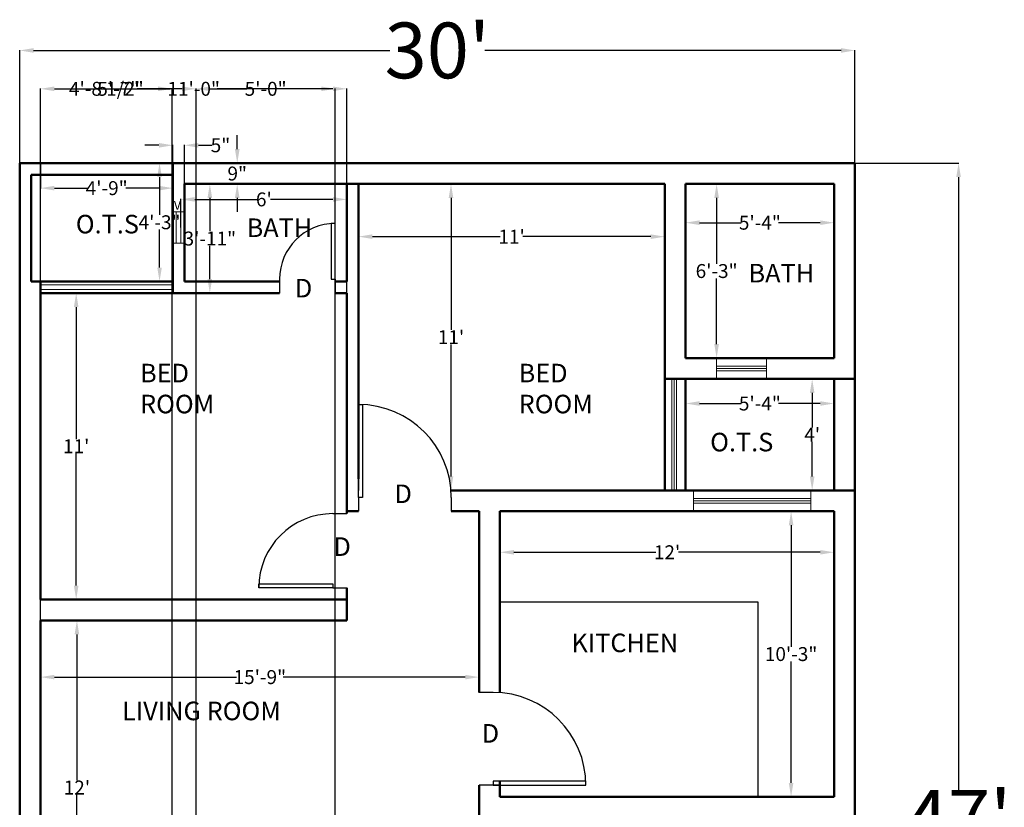
# Model space of a CAD drawing. Units: inches. Extents: x -251 to 272, y 511 to 1173.
# Tile 2 of 2: x -210 to 215, y 834 to 1173. Entities that reach past the tile are written whole.
import ezdxf

# ---------------------------------------------------------------- set-up
doc = ezdxf.new("R2010")
doc.units = ezdxf.units.IN
doc.header["$MEASUREMENT"] = 0
doc.layers.get('0').update_dxf_attribs({"color": 3})
for name, color, linetype, lineweight in [('A-AREA-IDEN', 20, 'Continuous', 25), ('A-FLOR-FIXT', 8, 'Continuous', 25), ('A-WALL', 7, 'Continuous', 50), ('dim', 2, 'Continuous', 18), ('door', 1, 'Continuous', 25), ('text', 20, 'Continuous', 18), ('window', 6, 'Continuous', 18)]:
    doc.layers.add(name, color=color, linetype=linetype, lineweight=lineweight)
doc.styles.get("Standard").update_dxf_attribs({"font": 'arial.ttf'})
doc.dimstyles.get("Standard").update_dxf_attribs({"dimtxt": 6, "dimasz": 6, "dimexe": 0.18, "dimexo": 0.0625, "dimgap": 0.09, "dimtad": 0, "dimtih": 1, "dimtoh": 1, "dimdec": 0, "dimzin": 0, "dimdsep": 46, "dimlunit": 3, "dimtxsty": 'Standard', "dimcen": 0.09, "dimadec": 0, "dimazin": 0, "dimtfac": 1, "dimtdec": 0, "dimtofl": 0, "dimtmove": 0, "dimatfit": 3, "dimfxl": 1, "dimtolj": 1, "dimtzin": 0, "dimarcsym": 0})

# ---------------------------------------------------------------- blocks, each defined once
blk = doc.blocks.new('*U2')
for p, q in [((-24, 0), (-24, -6)), ((0, 0), (0, -6))]:
    blk.add_line(p, q)
blk.add_lwpolyline([(0, 0), (0, 24), (-1.75, 24), (-1.75, 0)], close=True)
blk.add_arc((0, 0), 24, 90, 180)
blk = doc.blocks.new('*D3')
at = {"layer": 'Defpoints', "color": 0, "transparency": 16777216}
for p in [(-143.69, 1111.09), (-149.41, 1060.09), (-143.69, 1060.09)]:
    blk.add_point(p, dxfattribs=at)
at = {"layer": 'dim', "color": 0, "lineweight": -2, "transparency": 16777216}
for p, q in [((-143.75, 1111.09), (-149.59, 1111.09)), ((-149.41, 1105.09), (-149.41, 1088.74)), ((-149.41, 1066.09), (-149.41, 1082.43)), ((-143.75, 1060.09), (-149.59, 1060.09))]:
    blk.add_line(p, q, dxfattribs=at)
at = {"layer": 'dim', "color": 0, "transparency": 16777216}
for points in [[(-150.41, 1105.09), (-148.41, 1105.09), (-149.41, 1111.09)], [(-150.41, 1066.09), (-148.41, 1066.09), (-149.41, 1060.09)]]:
    blk.add_solid(points, dxfattribs=at)
at = {"layer": 'dim', "color": 0, "transparency": 16777216, "insert": (-149.41, 1085.59), "char_height": 6, "attachment_point": 5}
blk.add_mtext('\\A1;4\'-3"', dxfattribs=at)
blk = doc.blocks.new('*D4')
at = {"layer": 'Defpoints', "color": 0, "transparency": 16777216}
for p in [(-200.69, 1111.09), (-143.69, 1111.09), (-143.69, 1100.3)]:
    blk.add_point(p, dxfattribs=at)
at = {"layer": 'dim', "color": 0, "lineweight": -2, "transparency": 16777216}
for p, q in [((-200.69, 1111.02), (-200.69, 1100.12)), ((-143.69, 1111.02), (-143.69, 1100.12)), ((-194.69, 1100.3), (-180.37, 1100.3)), ((-149.69, 1100.3), (-164, 1100.3))]:
    blk.add_line(p, q, dxfattribs=at)
at = {"layer": 'dim', "color": 0, "transparency": 16777216}
for points in [[(-194.69, 1101.3), (-194.69, 1099.3), (-200.69, 1100.3)], [(-149.69, 1101.3), (-149.69, 1099.3), (-143.69, 1100.3)]]:
    blk.add_solid(points, dxfattribs=at)
at = {"layer": 'dim', "color": 0, "transparency": 16777216, "insert": (-172.19, 1100.3), "char_height": 6, "attachment_point": 5}
blk.add_mtext('\\A1;4\'-9"', dxfattribs=at)
blk = doc.blocks.new('*D5')
at = {"layer": 'Defpoints', "color": 0, "transparency": 16777216}
for p in [(-138.69, 1118.76), (-143.69, 1100.12), (-138.69, 1100.12)]:
    blk.add_point(p, dxfattribs=at)
at = {"layer": 'dim', "color": 0, "lineweight": -2, "transparency": 16777216}
for p, q in [((-149.69, 1118.76), (-155.69, 1118.76)), ((-143.69, 1100.19), (-143.69, 1118.94)), ((-138.69, 1100.19), (-138.69, 1118.94)), ((-132.69, 1118.76), (-126.69, 1118.76))]:
    blk.add_line(p, q, dxfattribs=at)
at = {"layer": 'dim', "color": 0, "transparency": 16777216}
for points in [[(-149.69, 1119.76), (-149.69, 1117.76), (-143.69, 1118.76)], [(-132.69, 1119.76), (-132.69, 1117.76), (-138.69, 1118.76)]]:
    blk.add_solid(points, dxfattribs=at)
at = {"layer": 'dim', "color": 0, "transparency": 16777216, "insert": (-123.15, 1118.76), "char_height": 6, "attachment_point": 5}
blk.add_mtext('\\A1;5"', dxfattribs=at)
blk = doc.blocks.new('*D6')
at = {"layer": 'Defpoints', "color": 0, "transparency": 16777216}
for p in [(-125.07, 1111.09), (-124.46, 1102.09), (-115.93, 1102.09)]:
    blk.add_point(p, dxfattribs=at)
at = {"layer": 'dim', "color": 0, "lineweight": -2, "transparency": 16777216}
for p, q in [((-115.93, 1117.09), (-115.93, 1123.09)), ((-125, 1111.09), (-115.75, 1111.09)), ((-124.39, 1102.09), (-115.75, 1102.09)), ((-115.93, 1096.09), (-115.93, 1090.09))]:
    blk.add_line(p, q, dxfattribs=at)
at = {"layer": 'dim', "color": 0, "transparency": 16777216}
for points in [[(-116.93, 1117.09), (-114.93, 1117.09), (-115.93, 1111.09)], [(-116.93, 1096.09), (-114.93, 1096.09), (-115.93, 1102.09)]]:
    blk.add_solid(points, dxfattribs=at)
at = {"layer": 'dim', "color": 0, "transparency": 16777216, "insert": (-115.93, 1106.59), "char_height": 6, "attachment_point": 5}
blk.add_mtext('\\A1;9"', dxfattribs=at)
blk = doc.blocks.new('*D7')
at = {"layer": 'Defpoints', "color": 0, "transparency": 16777216}
for p in [(-200.69, 1055.09), (-200.69, 923.09), (-185.34, 923.09)]:
    blk.add_point(p, dxfattribs=at)
at = {"layer": 'dim', "color": 0, "lineweight": -2, "transparency": 16777216}
for p, q in [((-200.63, 1055.09), (-185.16, 1055.09)), ((-185.34, 1049.09), (-185.34, 992.19)), ((-185.34, 929.09), (-185.34, 985.99)), ((-200.63, 923.09), (-185.16, 923.09))]:
    blk.add_line(p, q, dxfattribs=at)
at = {"layer": 'dim', "color": 0, "transparency": 16777216}
for points in [[(-186.34, 1049.09), (-184.34, 1049.09), (-185.34, 1055.09)], [(-186.34, 929.09), (-184.34, 929.09), (-185.34, 923.09)]]:
    blk.add_solid(points, dxfattribs=at)
at = {"layer": 'dim', "color": 0, "transparency": 16777216, "insert": (-185.34, 989.09), "char_height": 6, "attachment_point": 5}
blk.add_mtext("\\A1;11'", dxfattribs=at)
blk = doc.blocks.new('*U12')
for p, q in [((0, 0), (0, -6)), ((32, 0), (32, -6))]:
    blk.add_line(p, q)
blk.add_lwpolyline([(0, 0), (0, 32), (1.75, 32), (1.75, 0)], close=True)
blk.add_arc((0, 0), 32, 0, 90)
blk = doc.blocks.new('*U8')
for p, q in [((0, 0), (0, -6)), ((40, 0), (40, -6))]:
    blk.add_line(p, q)
blk.add_lwpolyline([(0, 0), (0, 40), (1.75, 40), (1.75, 0)], close=True)
blk.add_arc((0, 0), 40, 0, 90)
blk = doc.blocks.new('*D9')
at = {"layer": 'Defpoints', "color": 0, "transparency": 16777216}
for p in [(-68.69, 1095.45), (-140.22, 1083.32), (-68.69, 1083.32)]:
    blk.add_point(p, dxfattribs=at)
at = {"layer": 'dim', "color": 0, "lineweight": -2, "transparency": 16777216}
for p, q in [((-140.22, 1083.38), (-140.22, 1095.63)), ((-134.22, 1095.45), (-107.32, 1095.45)), ((-74.69, 1095.45), (-101.59, 1095.45)), ((-68.69, 1083.38), (-68.69, 1095.63))]:
    blk.add_line(p, q, dxfattribs=at)
at = {"layer": 'dim', "color": 0, "transparency": 16777216}
for points in [[(-134.22, 1096.45), (-134.22, 1094.45), (-140.22, 1095.45)], [(-74.69, 1096.45), (-74.69, 1094.45), (-68.69, 1095.45)]]:
    blk.add_solid(points, dxfattribs=at)
at = {"layer": 'dim', "color": 0, "transparency": 16777216, "insert": (-104.46, 1095.45), "char_height": 6, "attachment_point": 5}
blk.add_mtext("\\A1;6'", dxfattribs=at)
blk = doc.blocks.new('*D10')
at = {"layer": 'Defpoints', "color": 0, "transparency": 16777216}
for p in [(-127.74, 1102.09), (-127.74, 1102.09), (-127.74, 1055.09)]:
    blk.add_point(p, dxfattribs=at)
at = {"layer": 'dim', "color": 0, "lineweight": -2, "transparency": 16777216}
for p, q in [((-127.8, 1102.09), (-127.92, 1102.09)), ((-127.74, 1096.09), (-127.74, 1081.74)), ((-127.74, 1061.09), (-127.74, 1075.43)), ((-127.8, 1055.09), (-127.92, 1055.09))]:
    blk.add_line(p, q, dxfattribs=at)
at = {"layer": 'dim', "color": 0, "transparency": 16777216}
for points in [[(-128.74, 1096.09), (-126.74, 1096.09), (-127.74, 1102.09)], [(-128.74, 1061.09), (-126.74, 1061.09), (-127.74, 1055.09)]]:
    blk.add_solid(points, dxfattribs=at)
at = {"layer": 'dim', "color": 0, "transparency": 16777216, "insert": (-127.74, 1078.59), "char_height": 6, "attachment_point": 5}
blk.add_mtext('\\A1;3\'-11"', dxfattribs=at)
blk = doc.blocks.new('*D11')
at = {"layer": 'Defpoints', "color": 0, "transparency": 16777216}
for p in [(-63.69, 1102.09), (68.31, 1102.09), (68.31, 1079.4)]:
    blk.add_point(p, dxfattribs=at)
at = {"layer": 'dim', "color": 0, "lineweight": -2, "transparency": 16777216}
for p, q in [((-63.69, 1102.02), (-63.69, 1079.22)), ((68.31, 1102.02), (68.31, 1079.22)), ((-57.69, 1079.4), (-2.59, 1079.4)), ((62.31, 1079.4), (7.21, 1079.4))]:
    blk.add_line(p, q, dxfattribs=at)
at = {"layer": 'dim', "color": 0, "transparency": 16777216}
for points in [[(-57.69, 1080.4), (-57.69, 1078.4), (-63.69, 1079.4)], [(62.31, 1080.4), (62.31, 1078.4), (68.31, 1079.4)]]:
    blk.add_solid(points, dxfattribs=at)
at = {"layer": 'dim', "color": 0, "transparency": 16777216, "insert": (2.31, 1079.4), "char_height": 6, "attachment_point": 5}
blk.add_mtext("\\A1;11'", dxfattribs=at)
blk = doc.blocks.new('*D13')
at = {"layer": 'Defpoints', "color": 0, "transparency": 16777216}
for p in [(-0.19, 1102.09), (-23.8, 970.09), (-0.19, 970.09)]:
    blk.add_point(p, dxfattribs=at)
at = {"layer": 'dim', "color": 0, "lineweight": -2, "transparency": 16777216}
for p, q in [((-0.25, 1102.09), (-23.98, 1102.09)), ((-23.8, 1096.09), (-23.8, 1039.19)), ((-23.8, 976.09), (-23.8, 1032.99)), ((-0.25, 970.09), (-23.98, 970.09))]:
    blk.add_line(p, q, dxfattribs=at)
at = {"layer": 'dim', "color": 0, "transparency": 16777216}
for points in [[(-24.8, 1096.09), (-22.8, 1096.09), (-23.8, 1102.09)], [(-24.8, 976.09), (-22.8, 976.09), (-23.8, 970.09)]]:
    blk.add_solid(points, dxfattribs=at)
at = {"layer": 'dim', "color": 0, "transparency": 16777216, "insert": (-23.8, 1036.09), "char_height": 6, "attachment_point": 5}
blk.add_mtext("\\A1;11'", dxfattribs=at)
blk = doc.blocks.new('*D14')
at = {"layer": 'Defpoints', "color": 0, "transparency": 16777216}
for p in [(77.31, 1102.09), (77.31, 1027.09), (90.67, 1027.09)]:
    blk.add_point(p, dxfattribs=at)
at = {"layer": 'dim', "color": 0, "lineweight": -2, "transparency": 16777216}
for p, q in [((77.37, 1102.09), (90.85, 1102.09)), ((90.67, 1096.09), (90.67, 1067.74)), ((90.67, 1033.09), (90.67, 1061.43)), ((77.37, 1027.09), (90.85, 1027.09))]:
    blk.add_line(p, q, dxfattribs=at)
at = {"layer": 'dim', "color": 0, "transparency": 16777216}
for points in [[(89.67, 1096.09), (91.67, 1096.09), (90.67, 1102.09)], [(89.67, 1033.09), (91.67, 1033.09), (90.67, 1027.09)]]:
    blk.add_solid(points, dxfattribs=at)
at = {"layer": 'dim', "color": 0, "transparency": 16777216, "insert": (90.67, 1064.59), "char_height": 6, "attachment_point": 5}
blk.add_mtext('\\A1;6\'-3"', dxfattribs=at)
blk = doc.blocks.new('*D15')
at = {"layer": 'Defpoints', "color": 0, "transparency": 16777216}
for p in [(77.31, 1102.09), (141.31, 1102.09), (77.31, 1085.41)]:
    blk.add_point(p, dxfattribs=at)
at = {"layer": 'dim', "color": 0, "lineweight": -2, "transparency": 16777216}
for p, q in [((77.31, 1102.02), (77.31, 1085.23)), ((141.31, 1102.02), (141.31, 1085.23)), ((83.31, 1085.41), (101.25, 1085.41)), ((135.31, 1085.41), (117.38, 1085.41))]:
    blk.add_line(p, q, dxfattribs=at)
at = {"layer": 'dim', "color": 0, "transparency": 16777216}
for points in [[(83.31, 1086.41), (83.31, 1084.41), (77.31, 1085.41)], [(135.31, 1086.41), (135.31, 1084.41), (141.31, 1085.41)]]:
    blk.add_solid(points, dxfattribs=at)
at = {"layer": 'dim', "color": 0, "transparency": 16777216, "insert": (109.31, 1085.41), "char_height": 6, "attachment_point": 5}
blk.add_mtext('\\A1;5\'-4"', dxfattribs=at)
blk = doc.blocks.new('*D16')
at = {"layer": 'Defpoints', "color": 0, "transparency": 16777216}
for p in [(77.31, 1018.09), (141.31, 1018.09), (77.31, 1007.53)]:
    blk.add_point(p, dxfattribs=at)
at = {"layer": 'dim', "color": 0, "lineweight": -2, "transparency": 16777216}
for p, q in [((77.31, 1018.02), (77.31, 1007.35)), ((141.31, 1018.02), (141.31, 1007.35)), ((83.31, 1007.53), (101.25, 1007.53)), ((135.31, 1007.53), (117.38, 1007.53))]:
    blk.add_line(p, q, dxfattribs=at)
at = {"layer": 'dim', "color": 0, "transparency": 16777216}
for points in [[(83.31, 1008.53), (83.31, 1006.53), (77.31, 1007.53)], [(135.31, 1008.53), (135.31, 1006.53), (141.31, 1007.53)]]:
    blk.add_solid(points, dxfattribs=at)
at = {"layer": 'dim', "color": 0, "transparency": 16777216, "insert": (109.31, 1007.53), "char_height": 6, "attachment_point": 5}
blk.add_mtext('\\A1;5\'-4"', dxfattribs=at)
blk = doc.blocks.new('*D17')
at = {"layer": 'Defpoints', "color": 0, "transparency": 16777216}
for p in [(131.85, 1018.09), (141.31, 1018.09), (141.31, 970.09)]:
    blk.add_point(p, dxfattribs=at)
at = {"layer": 'dim', "color": 0, "lineweight": -2, "transparency": 16777216}
for p, q in [((141.25, 1018.09), (131.67, 1018.09)), ((131.85, 1012.09), (131.85, 997.18)), ((131.85, 976.09), (131.85, 991)), ((141.25, 970.09), (131.67, 970.09))]:
    blk.add_line(p, q, dxfattribs=at)
at = {"layer": 'dim', "color": 0, "transparency": 16777216}
for points in [[(130.85, 1012.09), (132.85, 1012.09), (131.85, 1018.09)], [(130.85, 976.09), (132.85, 976.09), (131.85, 970.09)]]:
    blk.add_solid(points, dxfattribs=at)
at = {"layer": 'dim', "color": 0, "transparency": 16777216, "insert": (131.85, 994.09), "char_height": 6, "attachment_point": 5}
blk.add_mtext("\\A1;4'", dxfattribs=at)
blk = doc.blocks.new('*U18')
for p, q in [((0, 0), (0, 6)), ((40, 0), (40, 6))]:
    blk.add_line(p, q)
blk.add_lwpolyline([(0, 0), (0, -40), (1.75, -40), (1.75, 0)], close=True)
blk.add_arc((0, 0), 40, 270, 0)
blk = doc.blocks.new('*D19')
at = {"layer": 'Defpoints', "color": 0, "transparency": 16777216}
for p in [(141.31, 961.09), (122.77, 838.09), (141.31, 838.09)]:
    blk.add_point(p, dxfattribs=at)
at = {"layer": 'dim', "color": 0, "lineweight": -2, "transparency": 16777216}
for p, q in [((141.25, 961.09), (122.59, 961.09)), ((122.77, 955.09), (122.77, 902.74)), ((122.77, 844.09), (122.77, 896.43)), ((141.25, 838.09), (122.59, 838.09))]:
    blk.add_line(p, q, dxfattribs=at)
at = {"layer": 'dim', "color": 0, "transparency": 16777216}
for points in [[(121.77, 955.09), (123.77, 955.09), (122.77, 961.09)], [(121.77, 844.09), (123.77, 844.09), (122.77, 838.09)]]:
    blk.add_solid(points, dxfattribs=at)
at = {"layer": 'dim', "color": 0, "transparency": 16777216, "insert": (122.77, 899.59), "char_height": 6, "attachment_point": 5}
blk.add_mtext('\\A1;10\'-3"', dxfattribs=at)
blk = doc.blocks.new('*D20')
at = {"layer": 'Defpoints', "color": 0, "transparency": 16777216}
for p in [(-2.69, 961.09), (141.31, 961.09), (141.31, 943.44)]:
    blk.add_point(p, dxfattribs=at)
at = {"layer": 'dim', "color": 0, "lineweight": -2, "transparency": 16777216}
for p, q in [((-2.69, 961.02), (-2.69, 943.26)), ((141.31, 961.02), (141.31, 943.26)), ((3.31, 943.44), (64.41, 943.44)), ((135.31, 943.44), (74.21, 943.44))]:
    blk.add_line(p, q, dxfattribs=at)
at = {"layer": 'dim', "color": 0, "transparency": 16777216}
for points in [[(3.31, 944.44), (3.31, 942.44), (-2.69, 943.44)], [(135.31, 944.44), (135.31, 942.44), (141.31, 943.44)]]:
    blk.add_solid(points, dxfattribs=at)
at = {"layer": 'dim', "color": 0, "transparency": 16777216, "insert": (69.31, 943.44), "char_height": 6, "attachment_point": 5}
blk.add_mtext("\\A1;12'", dxfattribs=at)
blk = doc.blocks.new('*D36')
at = {"layer": 'Defpoints', "color": 0, "transparency": 16777216}
for p in [(-200.69, 914.09), (-200.69, 770.09), (-185.02, 770.09)]:
    blk.add_point(p, dxfattribs=at)
at = {"layer": 'dim', "color": 0, "lineweight": -2, "transparency": 16777216}
for p, q in [((-200.63, 914.09), (-184.84, 914.09)), ((-185.02, 908.09), (-185.02, 845.19)), ((-185.02, 776.09), (-185.02, 838.99)), ((-200.63, 770.09), (-184.84, 770.09))]:
    blk.add_line(p, q, dxfattribs=at)
at = {"layer": 'dim', "color": 0, "transparency": 16777216}
for points in [[(-186.02, 908.09), (-184.02, 908.09), (-185.02, 914.09)], [(-186.02, 776.09), (-184.02, 776.09), (-185.02, 770.09)]]:
    blk.add_solid(points, dxfattribs=at)
at = {"layer": 'dim', "color": 0, "transparency": 16777216, "insert": (-185.02, 842.09), "char_height": 6, "attachment_point": 5}
blk.add_mtext("\\A1;12'", dxfattribs=at)
blk = doc.blocks.new('*D37')
at = {"layer": 'Defpoints', "color": 0, "transparency": 16777216}
for p in [(-200.69, 914.09), (-11.69, 914.09), (-11.69, 889.67)]:
    blk.add_point(p, dxfattribs=at)
at = {"layer": 'dim', "color": 0, "lineweight": -2, "transparency": 16777216}
for p, q in [((-200.69, 914.02), (-200.69, 889.49)), ((-11.69, 914.02), (-11.69, 889.49)), ((-194.69, 889.67), (-116.3, 889.67)), ((-17.69, 889.67), (-96.07, 889.67))]:
    blk.add_line(p, q, dxfattribs=at)
at = {"layer": 'dim', "color": 0, "transparency": 16777216}
for points in [[(-194.69, 890.67), (-194.69, 888.67), (-200.69, 889.67)], [(-17.69, 890.67), (-17.69, 888.67), (-11.69, 889.67)]]:
    blk.add_solid(points, dxfattribs=at)
at = {"layer": 'dim', "color": 0, "transparency": 16777216, "insert": (-106.19, 889.67), "char_height": 6, "attachment_point": 5}
blk.add_mtext('\\A1;15\'-9"', dxfattribs=at)
blk = doc.blocks.new('*D38')
at = {"layer": 'Defpoints', "color": 0, "transparency": 16777216}
for p in [(150.31, 1111.09), (150.31, 547.09), (194.95, 547.09)]:
    blk.add_point(p, dxfattribs=at)
at = {"layer": 'dim', "color": 0, "lineweight": -2, "transparency": 16777216}
for p, q in [((150.37, 1111.09), (195.13, 1111.09)), ((194.95, 1105.09), (194.95, 841.18)), ((194.95, 553.09), (194.95, 817)), ((150.37, 547.09), (195.13, 547.09))]:
    blk.add_line(p, q, dxfattribs=at)
at = {"layer": 'dim', "color": 0, "transparency": 16777216}
for points in [[(193.95, 1105.09), (195.95, 1105.09), (194.95, 1111.09)], [(193.95, 553.09), (195.95, 553.09), (194.95, 547.09)]]:
    blk.add_solid(points, dxfattribs=at)
at = {"layer": 'dim', "color": 0, "transparency": 16777216, "insert": (194.95, 829.09), "char_height": 6, "attachment_point": 5}
blk.add_mtext("\\A1;{\\H4x;47'}", dxfattribs=at)
blk = doc.blocks.new('*D39')
at = {"layer": 'Defpoints', "color": 0, "transparency": 16777216}
for p in [(150.31, 1159.61), (-209.69, 1111.09), (150.31, 1111.09)]:
    blk.add_point(p, dxfattribs=at)
at = {"layer": 'dim', "color": 0, "lineweight": -2, "transparency": 16777216}
for p, q in [((-209.69, 1111.15), (-209.69, 1159.79)), ((-203.69, 1159.61), (-50.14, 1159.61)), ((144.31, 1159.61), (-9.24, 1159.61)), ((150.31, 1111.15), (150.31, 1159.79))]:
    blk.add_line(p, q, dxfattribs=at)
at = {"layer": 'dim', "color": 0, "transparency": 16777216}
for points in [[(-203.69, 1160.61), (-203.69, 1158.61), (-209.69, 1159.61)], [(144.31, 1160.61), (144.31, 1158.61), (150.31, 1159.61)]]:
    blk.add_solid(points, dxfattribs=at)
at = {"layer": 'dim', "color": 0, "transparency": 16777216, "insert": (-29.69, 1159.61), "char_height": 6, "attachment_point": 5}
blk.add_mtext("\\A1;{\\H4x;30'}", dxfattribs=at)
blk = doc.blocks.new('*D47')
at = {"layer": 'Defpoints', "color": 0, "transparency": 16777216}
for p in [(-144.01, 1143.09), (-200.69, 761.09), (-144.01, 761.09)]:
    blk.add_point(p, dxfattribs=at)
at = {"layer": 'dim', "color": 0, "lineweight": -2, "transparency": 16777216}
for p, q in [((-200.69, 761.15), (-200.69, 1143.27)), ((-194.69, 1143.09), (-187.52, 1143.09)), ((-150.01, 1143.09), (-157.17, 1143.09)), ((-144.01, 761.15), (-144.01, 1143.27))]:
    blk.add_line(p, q, dxfattribs=at)
at = {"layer": 'dim', "color": 0, "transparency": 16777216}
for points in [[(-194.69, 1144.09), (-194.69, 1142.09), (-200.69, 1143.09)], [(-150.01, 1144.09), (-150.01, 1142.09), (-144.01, 1143.09)]]:
    blk.add_solid(points, dxfattribs=at)
at = {"layer": 'dim', "color": 0, "transparency": 16777216, "insert": (-172.35, 1143.09), "char_height": 6, "attachment_point": 5}
blk.add_mtext('\\A1;4\'-8 1/2"', dxfattribs=at)
blk = doc.blocks.new('*D48')
at = {"layer": 'Defpoints', "color": 0, "transparency": 16777216}
for p in [(-68.69, 1143.09), (-200.69, 1055.09), (-68.69, 1055.09)]:
    blk.add_point(p, dxfattribs=at)
at = {"layer": 'dim', "color": 0, "lineweight": -2, "transparency": 16777216}
for p, q in [((-200.69, 1055.15), (-200.69, 1143.27)), ((-194.69, 1143.09), (-144.8, 1143.09)), ((-74.69, 1143.09), (-124.57, 1143.09)), ((-68.69, 1055.15), (-68.69, 1143.27))]:
    blk.add_line(p, q, dxfattribs=at)
at = {"layer": 'dim', "color": 0, "transparency": 16777216}
for points in [[(-194.69, 1144.09), (-194.69, 1142.09), (-200.69, 1143.09)], [(-74.69, 1144.09), (-74.69, 1142.09), (-68.69, 1143.09)]]:
    blk.add_solid(points, dxfattribs=at)
at = {"layer": 'dim', "color": 0, "transparency": 16777216, "insert": (-134.69, 1143.09), "char_height": 6, "attachment_point": 5}
blk.add_mtext('\\A1;11\'-0"', dxfattribs=at)
blk = doc.blocks.new('*D49')
at = {"layer": 'Defpoints', "color": 0, "transparency": 16777216}
for p in [(-73.69, 1143.09), (-133.69, 770.09), (-73.69, 770.09)]:
    blk.add_point(p, dxfattribs=at)
at = {"layer": 'dim', "color": 0, "lineweight": -2, "transparency": 16777216}
for p, q in [((-133.69, 770.15), (-133.69, 1143.27)), ((-127.69, 1143.09), (-111.75, 1143.09)), ((-79.69, 1143.09), (-95.62, 1143.09)), ((-73.69, 770.15), (-73.69, 1143.27))]:
    blk.add_line(p, q, dxfattribs=at)
at = {"layer": 'dim', "color": 0, "transparency": 16777216}
for points in [[(-127.69, 1144.09), (-127.69, 1142.09), (-133.69, 1143.09)], [(-79.69, 1144.09), (-79.69, 1142.09), (-73.69, 1143.09)]]:
    blk.add_solid(points, dxfattribs=at)
at = {"layer": 'dim', "color": 0, "transparency": 16777216, "insert": (-103.69, 1143.09), "char_height": 6, "attachment_point": 5}
blk.add_mtext('\\A1;5\'-0"', dxfattribs=at)
blk = doc.blocks.new('*D50')
at = {"layer": 'Defpoints', "color": 0, "transparency": 16777216}
for p in [(-133.69, 1143.09), (-200.69, 770.09), (-133.69, 770.09)]:
    blk.add_point(p, dxfattribs=at)
at = {"layer": 'dim', "color": 0, "lineweight": -2, "transparency": 16777216}
for p, q in [((-200.69, 770.15), (-200.69, 1143.27)), ((-194.69, 1143.09), (-175.25, 1143.09)), ((-139.69, 1143.09), (-159.12, 1143.09)), ((-133.69, 770.15), (-133.69, 1143.27))]:
    blk.add_line(p, q, dxfattribs=at)
at = {"layer": 'dim', "color": 0, "transparency": 16777216}
for points in [[(-194.69, 1144.09), (-194.69, 1142.09), (-200.69, 1143.09)], [(-139.69, 1144.09), (-139.69, 1142.09), (-133.69, 1143.09)]]:
    blk.add_solid(points, dxfattribs=at)
at = {"layer": 'dim', "color": 0, "transparency": 16777216, "insert": (-167.19, 1143.09), "char_height": 6, "attachment_point": 5}
blk.add_mtext('\\A1;5\'-7"', dxfattribs=at)

msp = doc.modelspace()

# ---------------------------------------------------------------- linework, layer by layer
at = {"layer": 'A-FLOR-FIXT'}
for p, q in [((-2.69, 961.09), (-2.69, 922.03)), ((-2.69, 922.03), (108.43, 922.03)), ((108.43, 922.03), (108.43, 838.09))]:
    msp.add_line(p, q, dxfattribs=at)
at = {"layer": 'A-WALL'}
for p, q in [((-209.69, 1111.09), (150.31, 1111.09)), ((-209.69, 547.09), (-209.69, 1111.09)), ((-143.69, 1111.09), (-143.69, 1059.71)), ((150.31, 1111.09), (150.31, 547.09)), ((-204.69, 1106.09), (-143.69, 1106.09)), ((-204.69, 1060.09), (-204.69, 1106.09)), ((-138.69, 1102.09), (-138.69, 1060.09)), ((-68.69, 1102.09), (58.31, 1102.09)), ((-68.69, 1060.09), (-68.69, 1102.09)), ((-68.69, 1102.09), (68.31, 1102.09)), ((-68.69, 1060.09), (-68.69, 1102.09)), ((-63.69, 975.09), (-63.69, 1102.09)), ((68.31, 970.09), (68.31, 1102.09)), ((77.31, 1102.09), (141.31, 1102.09)), ((77.31, 1027.09), (77.31, 1102.09)), ((77.31, 1027.09), (77.31, 1102.09)), ((141.31, 1102.09), (141.31, 1027.09)), ((-143.69, 1060.09), (-204.69, 1060.09)), ((-200.69, 923.09), (-200.69, 1060.09)), ((-143.69, 1059.71), (-143.69, 1055.09)), ((-97.69, 1060.09), (-138.69, 1060.09)), ((-68.69, 1060.09), (-73.69, 1060.09)), ((-143.69, 1055.09), (-200.69, 1055.09)), ((-97.69, 1055.09), (-143.69, 1055.09)), ((-68.69, 1055.09), (-73.69, 1055.09)), ((-68.69, 960.09), (-68.69, 1055.09)), ((141.31, 1027.09), (77.31, 1027.09)), ((68.31, 1018.09), (150.31, 1018.09)), ((77.31, 970.09), (77.31, 1018.09)), ((141.31, 1018.09), (77.31, 1018.09)), ((77.31, 970.09), (77.31, 1018.09)), ((141.31, 1018.09), (141.31, 970.09)), ((-68.69, 968.09), (-68.69, 970.09)), ((150.31, 970.09), (-23.8, 970.09)), ((-63.69, 961.09), (-68.69, 961.09)), ((-11.69, 961.09), (-23.69, 961.09)), ((-11.69, 961.09), (-11.69, 883.09)), ((141.31, 961.09), (-2.69, 961.09)), ((141.31, 961.09), (-2.69, 961.09)), ((-2.69, 961.09), (-2.69, 882.97)), ((141.31, 961.09), (141.31, 838.09)), ((141.31, 838.09), (141.31, 961.09)), ((-68.69, 914.09), (-68.69, 928.09)), ((-68.69, 923.09), (-200.69, 923.09)), ((-68.69, 914.09), (-200.69, 914.09)), ((-200.69, 914.09), (-68.69, 914.09)), ((-200.69, 770.09), (-200.69, 914.09)), ((-200.69, 770.09), (-200.69, 914.09)), ((-11.69, 914.09), (-11.69, 883.09)), ((-2.69, 844.84), (-2.69, 838.09)), ((-11.69, 843.09), (-11.69, 829.09)), ((-11.69, 843.09), (-11.69, 824.09)), ((-2.69, 838.09), (141.31, 838.09))]:
    msp.add_line(p, q, dxfattribs=at)
msp.add_lwpolyline([(-138.69, 1102.09), (-68.69, 1102.09)], dxfattribs=at)
at = {"layer": 'door'}
for p, q in [((-73.69, 1060.09), (-73.69, 1055.09)), ((-63.69, 975.09), (-63.69, 970.09)), ((-2.69, 843.09), (-11.69, 843.09))]:
    msp.add_line(p, q, dxfattribs=at)
at = {"layer": 'window'}
for p, q in [((-143.83, 1090.02), (-138.69, 1090.02)), ((-142.26, 1090.01), (-142.19, 1076.61)), ((-140.26, 1090.02), (-140.19, 1076.62)), ((-143.69, 1076.62), (-138.69, 1076.62)), ((-143.69, 1058.6), (-200.69, 1058.6)), ((-143.69, 1056.6), (-200.69, 1056.6)), ((90.67, 1027.09), (90.67, 1018.09)), ((112.15, 1027.09), (112.15, 1018.09)), ((90.67, 1023.59), (112.15, 1023.59)), ((90.67, 1022.59), (112.15, 1022.59)), ((90.67, 1021.59), (112.15, 1021.59)), ((71.42, 1018.09), (71.42, 970.09)), ((72.42, 1018.09), (72.42, 970.09)), ((73.42, 1018.09), (73.42, 970.09)), ((80.77, 970.09), (80.77, 961.09)), ((131.23, 970.09), (131.23, 961.09)), ((80.77, 966.59), (131.23, 966.59)), ((80.77, 965.59), (131.23, 965.59)), ((80.77, 964.59), (131.23, 964.59))]:
    msp.add_line(p, q, dxfattribs=at)

# ---------------------------------------------------------------- block references
at = {"layer": 'door'}
for name, p in [('*U2', (-73.69, 1061.09)), ('*U8', (-63.69, 967.09))]:
    msp.add_blockref(name, p, dxfattribs=at)
at = {"layer": 'door', "rotation": 90}
for name, p in [('*U12', (-74.69, 928.09)), ('*U18', (-5.69, 843.09))]:
    msp.add_blockref(name, p, dxfattribs=at)

# ---------------------------------------------------------------- texts
at = {"layer": 'A-AREA-IDEN', "char_height": 8, "attachment_point": 1}
for s, width, insert in [('O.T.S', 25.4401, (-185.5, 1088.8)), ('BATH', 36.4399, (-111.88, 1087.23)), ('BATH', 36.4399, (104.42, 1067.67)), ('BED ROOM', 53.8549, (-157.82, 1024.63)), ('BED ROOM', 53.8549, (5.35, 1024.63)), ('O.T.S', 25.4401, (87.89, 994.91)), ('KITCHEN', 50.0499, (28.08, 908.41)), ('LIVING ROOM', 74.5529, (-165.58, 879.09))]:
    msp.add_mtext_dynamic_manual_height_columns(s, width=width, gutter_width=1, heights=[0], dxfattribs=dict(at, insert=insert))
at = {"layer": 'text', "attachment_point": 1}
for s, width, gutter_width, insert, char_height in [('V', 0.9908, 0.469, (-143.2, 1094.73), 3.75), ('D', 6.3802, 1, (-91.09, 1061.2), 8), ('D', 6.3802, 1, (-48.16, 972.63), 8), ('D', 6.3802, 1, (-74.48, 949.88), 8), ('D', 6.3802, 1, (-10.57, 869.43), 8)]:
    msp.add_mtext_dynamic_manual_height_columns(s, width=width, gutter_width=gutter_width, heights=[0], dxfattribs=dict(at, insert=insert, char_height=char_height))

# ---------------------------------------------------------------- dimensions: what is measured, and where the dimension line sits
at = {"layer": 'dim'}
dim = msp.add_linear_dim(base=(150.31, 1159.61), p1=(-209.69, 1111.09), p2=(150.31, 1111.09), text='{\\H4x;<>}', dimstyle='Standard', override={"dimclrd": 0, "dimclre": 0, "dimclrt": 0}, dxfattribs=at)
dim.commit()
dim.dimension.update_dxf_attribs({"geometry": '*D39', "text_midpoint": (-29.69, 1159.61)})
for base, p1, p2, override, picture, middle in [((-144.01, 1143.09), (-200.69, 761.09), (-144.01, 761.09), {"dimdec": 1, "dimlfac": 1, "dimrnd": 0, "dimzin": 1, "dimdsep": 46, "dimlunit": 4, "dimfrac": 2}, '*D47', (-172.35, 1143.09)), ((-68.69, 1143.09), (-200.69, 1055.09), (-68.69, 1055.09), {"dimdec": 1, "dimlfac": 1, "dimrnd": 0, "dimzin": 1, "dimdsep": 46, "dimlunit": 4, "dimfrac": 2}, '*D48', (-134.69, 1143.09)), ((-133.69, 1143.09), (-200.69, 770.09), (-133.69, 770.09), {"dimdec": 1, "dimlfac": 1, "dimrnd": 0, "dimzin": 1, "dimdsep": 46, "dimlunit": 4, "dimfrac": 2}, '*D50', (-167.19, 1143.09)), ((-73.69, 1143.09), (-133.69, 770.09), (-73.69, 770.09), {"dimdec": 1, "dimlfac": 1, "dimrnd": 0, "dimzin": 1, "dimdsep": 46, "dimlunit": 4, "dimfrac": 2}, '*D49', (-103.69, 1143.09)), ((-138.69, 1118.76), (-143.69, 1100.12), (-138.69, 1100.12), {"dimclrd": 0, "dimclre": 0, "dimclrt": 0}, '*D5', (-123.15, 1118.76)), ((-143.69, 1100.3), (-200.69, 1111.09), (-143.69, 1111.09), {"dimclrd": 0, "dimclre": 0, "dimclrt": 0}, '*D4', (-172.19, 1100.3)), ((-68.69, 1095.45), (-140.22, 1083.32), (-68.69, 1083.32), {"dimclrd": 0, "dimclre": 0, "dimclrt": 0}, '*D9', (-104.46, 1095.45)), ((68.31, 1079.4), (-63.69, 1102.09), (68.31, 1102.09), {"dimclrd": 0, "dimclre": 0, "dimclrt": 0}, '*D11', (2.31, 1079.4)), ((77.31, 1085.41), (141.31, 1102.09), (77.31, 1102.09), {"dimclrd": 0, "dimclre": 0, "dimclrt": 0}, '*D15', (109.31, 1085.41)), ((77.31, 1007.53), (141.31, 1018.09), (77.31, 1018.09), {"dimclrd": 0, "dimclre": 0, "dimclrt": 0}, '*D16', (109.31, 1007.53)), ((141.31, 943.44), (-2.69, 961.09), (141.31, 961.09), {"dimclrd": 0, "dimclre": 0, "dimclrt": 0}, '*D20', (69.31, 943.44)), ((-11.69, 889.67), (-200.69, 914.09), (-11.69, 914.09), {"dimclrd": 0, "dimclre": 0, "dimclrt": 0}, '*D37', (-106.19, 889.67))]:
    dim = msp.add_linear_dim(base=base, p1=p1, p2=p2, dimstyle='Standard', override=override, dxfattribs=at)
    dim.commit()
    dim.dimension.update_dxf_attribs({"geometry": picture, "text_midpoint": middle})
for base, p1, p2, picture, middle in [((-115.93, 1102.09), (-125.07, 1111.09), (-124.46, 1102.09), '*D6', (-115.93, 1106.59)), ((-149.41, 1060.09), (-143.69, 1111.09), (-143.69, 1060.09), '*D3', (-149.41, 1085.59)), ((-127.74, 1102.09), (-127.74, 1055.09), (-127.74, 1102.09), '*D10', (-127.74, 1078.59)), ((-23.8, 970.09), (-0.19, 1102.09), (-0.19, 970.09), '*D13', (-23.8, 1036.09)), ((90.67, 1027.09), (77.31, 1102.09), (77.31, 1027.09), '*D14', (90.67, 1064.59)), ((-185.34, 923.09), (-200.69, 1055.09), (-200.69, 923.09), '*D7', (-185.34, 989.09)), ((131.85, 1018.09), (141.31, 970.09), (141.31, 1018.09), '*D17', (131.85, 994.09)), ((122.77, 838.09), (141.31, 961.09), (141.31, 838.09), '*D19', (122.77, 899.59)), ((-185.02, 770.09), (-200.69, 914.09), (-200.69, 770.09), '*D36', (-185.02, 842.09))]:
    dim = msp.add_linear_dim(base=base, p1=p1, p2=p2, angle=90, dimstyle='Standard', override={"dimclrd": 0, "dimclre": 0, "dimclrt": 0}, dxfattribs=at)
    dim.commit()
    dim.dimension.update_dxf_attribs({"geometry": picture, "text_midpoint": middle})
dim = msp.add_linear_dim(base=(194.95, 547.09), p1=(150.31, 1111.09), p2=(150.31, 547.09), angle=90, text='{\\H4x;<>}', dimstyle='Standard', override={"dimclrd": 0, "dimclre": 0, "dimclrt": 0}, dxfattribs=at)
dim.commit()
dim.dimension.update_dxf_attribs({"geometry": '*D38', "text_midpoint": (194.95, 829.09)})

doc.saveas('drawing.dxf')
